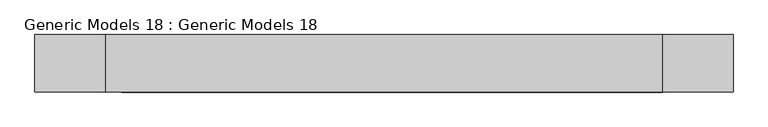
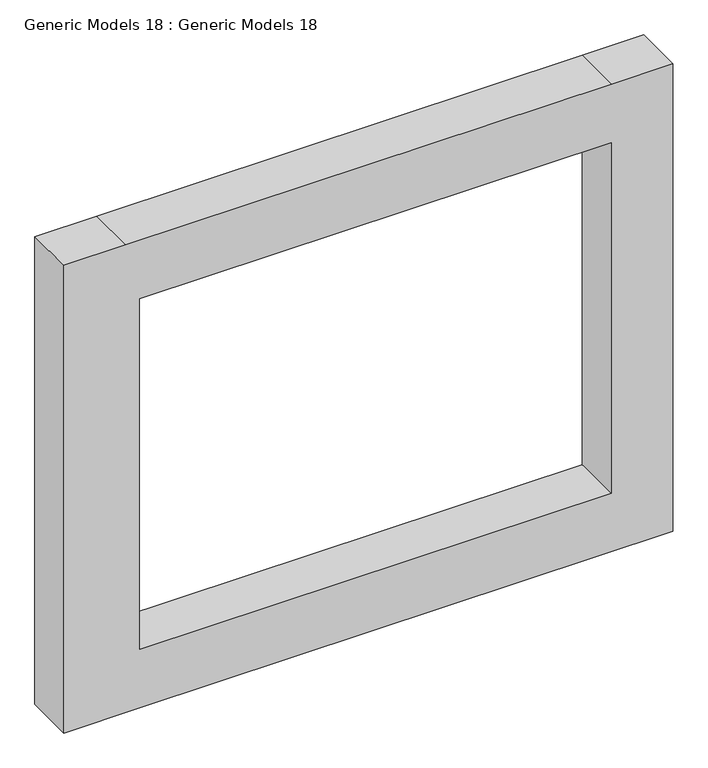
"""IFC4 building model written with IfcOpenShell, lengths in millimetres: proxy geometry, Generic Models 18 : Generic Models 18."""

from ifc_helpers import new_model, si_unit, frame, origin, place, context, project, spatial, polyline, outline, extrude, source, transform, mapped, element, save


def generic_models_18_generic_models_18_97eb84db(model_context):
    return source(origin(), model_context, "Body", "SweptSolid", [
        extrude(outline(polyline([(2743.2, -530.4536806), (2743.2, -2924.4036806), (2743.2, -3229.2036806), (304.8, -3229.2036806), (304.8, -2854.5536806), (304.8, -225.6536806), (609.6, -225.6536806), (2743.2, -225.6536806), (2743.2, -530.4536806)]), holes=[polyline([(2438.4, -530.4536806), (609.6, -530.4536806), (609.6, -2854.5536806), (2438.4, -2854.5536806), (2438.4, -530.4536806)])]), frame((0.0, -3966.662639, 0.0), z_axis=(0.0, 1.0, 0.0), x_axis=(0.0, 0.0, 1.0)), (0.0, 0.0, 1.0), 247.5353288),
    ])


if __name__ == "__main__":
    model = new_model("IFC4")
    model_context = context("Model", 3, world=origin())
    ifc_project = project(units=[si_unit("LENGTHUNIT", "METRE", prefix="MILLI")], contexts=[model_context])
    site = spatial("IfcSite", under=ifc_project)
    building = spatial("IfcBuilding", under=site)
    placement = place(None, origin())
    generic_models_18_generic_models_18_shape = generic_models_18_generic_models_18_97eb84db(model_context)
    element("IfcBuildingElementProxy", 1, Name="Generic Models 18 : Generic Models 18", ObjectType="Generic Models 18 : Generic Models 18", at=placement, inside=building, context=model_context, shape_type="MappedRepresentation", body=[
        mapped(generic_models_18_generic_models_18_shape, transform((0.0, 0.0, 0.0), x_axis=(1.0, 0.0, 0.0), y_axis=(0.0, 1.0, 0.0), z_axis=(0.0, 0.0, 1.0))),
    ])
    save(model, "model.ifc")

# Revit data of these elements
# Element 1 (IfcBuildingElementProxy, "Generic Models 18 : Generic Models 18")
#   Materials on its faces: "exterior wall"
# Materials
#   "exterior wall": class "Generic", colour RGB 215 217 121, transparency 0, Cost = 0
